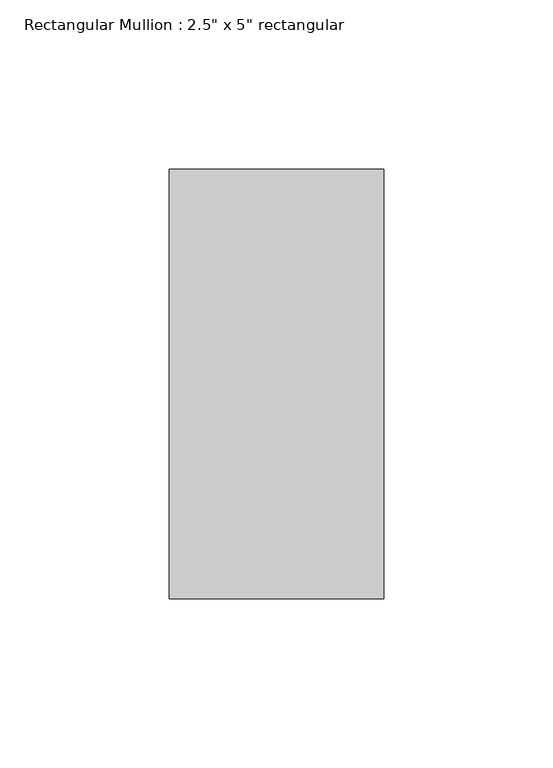
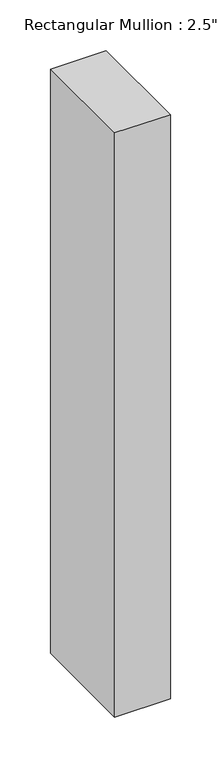
"""IFC4 building model written with IfcOpenShell, lengths in millimetres: member geometry."""

from ifc_helpers import new_model, si_unit, frame, origin, place, context, project, spatial, polyline, outline, extrude, source, transform, mapped, element, save


def member_6f814c25(model_context):
    return source(origin(), model_context, "Body", "SweptSolid", [
        extrude(outline(polyline([(0.0, 63.5), (0.0, -63.5), (-63.5, -63.5), (-63.5, 63.5), (0.0, 63.5)])), frame((0.0, 0.0, -704.4785299), z_axis=(0.0, 0.0, 1.0), x_axis=(1.0, 0.0, 0.0)), (0.0, 0.0, 1.0), 704.4785299),
    ])


if __name__ == "__main__":
    model = new_model("IFC4")
    model_context = context("Model", 3, world=origin())
    ifc_project = project(units=[si_unit("LENGTHUNIT", "METRE", prefix="MILLI")], contexts=[model_context])
    site = spatial("IfcSite", under=ifc_project)
    building = spatial("IfcBuilding", under=site)
    placement = place(None, origin())
    member_shape = member_6f814c25(model_context)
    element("IfcMember", 1, ObjectType="Rectangular Mullion : 2.5\" x 5\" rectangular", at=placement, inside=building, context=model_context, shape_type="MappedRepresentation", body=[
        mapped(member_shape, transform((0.0, 0.0, 0.0), x_axis=(1.0, 0.0, 0.0), y_axis=(0.0, 1.0, 0.0), z_axis=(0.0, 0.0, 1.0))),
    ])
    save(model, "model.ifc")

# Revit data of these elements
# Type "Rectangular Mullion : 2.5\" x 5\" rectangular"
#   built-in parameter 1007304 = 0.416667 (stored number, unit not read)
#   built-in parameter 1007301 = 0.104167 (stored number, unit not read)
#   built-in parameter 1007300 = 0.104167 (stored number, unit not read)
# Element 1 (IfcMember, "Rectangular Mullion : 2.5\" x 5\" rectangular")
#   Materials on its faces: "Aluminum"
# Materials
#   "Aluminum": class "Metal", colour RGB 247 247 247, transparency 0, Description = "Aluminum 6061", Cost = 0
